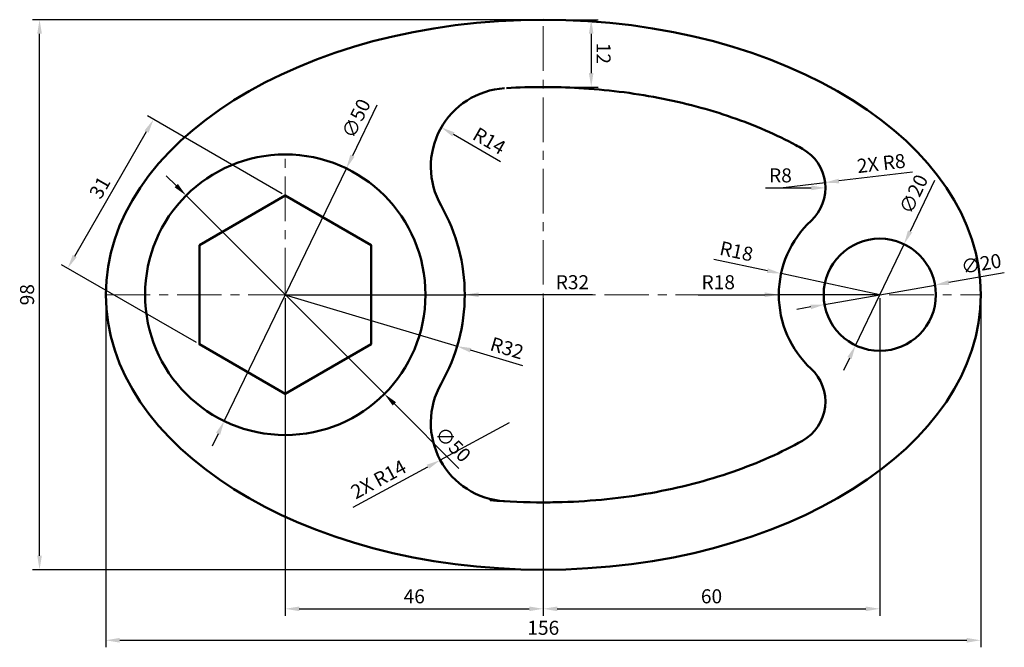
# Model space of a CAD drawing. Units: millimetres. Extents: x 1633 to 1808, y 1205 to 1317.
import ezdxf

# ---------------------------------------------------------------- set-up
doc = ezdxf.new("R2010")
doc.units = ezdxf.units.MM
doc.linetypes.add('CENTER', pattern=[50.8, 31.75, -6.35, 6.35, -6.35])
for name, color, linetype, lineweight in [('M-CNTR', 4, 'CENTER', 18), ('M-DIMS', 2, 'Continuous', 25), ('M-OUTL', 7, 'Continuous', 50)]:
    doc.layers.add(name, color=color, linetype=linetype, lineweight=lineweight)
doc.styles.get("Standard").update_dxf_attribs({"font": 'arial.ttf'})
doc.dimstyles.new('ISO-25', dxfattribs={"dimtxt": 2.5, "dimasz": 2.5, "dimexe": 1.25, "dimexo": 0.625, "dimtad": 1, "dimtxsty": 'Standard', "dimcen": 2.5, "dimadec": 0, "dimazin": 0, "dimtfac": 1, "dimtmove": 0, "dimatfit": 3, "dimfxl": 1, "dimarcsym": 0})

# ---------------------------------------------------------------- blocks, each defined once
blk = doc.blocks.new('*D1')
at = {"layer": 'Defpoints', "color": 0, "transparency": 16777216}
for p in [(1680.07, 1267.86), (1726.07, 1267.86), (1726.07, 1211.9)]:
    blk.add_point(p, dxfattribs=at)
at = {"layer": 'M-DIMS', "color": 0, "lineweight": -2, "transparency": 16777216}
for p, q in [((1680.07, 1267.23), (1680.07, 1210.65)), ((1726.07, 1267.23), (1726.07, 1210.65)), ((1682.57, 1211.9), (1723.57, 1211.9))]:
    blk.add_line(p, q, dxfattribs=at)
at = {"layer": 'M-DIMS', "color": 0, "transparency": 16777216}
for points in [[(1682.57, 1212.31), (1682.57, 1211.48), (1680.07, 1211.9)], [(1723.57, 1212.31), (1723.57, 1211.48), (1726.07, 1211.9)]]:
    blk.add_solid(points, dxfattribs=at)
at = {"layer": 'M-DIMS', "color": 0, "transparency": 16777216, "insert": (1703.07, 1213.8), "char_height": 2.5, "attachment_point": 5}
blk.add_mtext('46', dxfattribs=at)
blk = doc.blocks.new('*D2')
at = {"layer": 'Defpoints', "color": 0, "transparency": 16777216}
for p in [(1726.07, 1267.86), (1786.07, 1267.86), (1786.07, 1211.9)]:
    blk.add_point(p, dxfattribs=at)
at = {"layer": 'M-DIMS', "color": 0, "lineweight": -2, "transparency": 16777216}
for p, q in [((1726.07, 1267.23), (1726.07, 1210.65)), ((1786.07, 1267.23), (1786.07, 1210.65)), ((1728.57, 1211.9), (1783.57, 1211.9))]:
    blk.add_line(p, q, dxfattribs=at)
at = {"layer": 'M-DIMS', "color": 0, "transparency": 16777216}
for points in [[(1728.57, 1212.31), (1728.57, 1211.48), (1726.07, 1211.9)], [(1783.57, 1212.31), (1783.57, 1211.48), (1786.07, 1211.9)]]:
    blk.add_solid(points, dxfattribs=at)
at = {"layer": 'M-DIMS', "color": 0, "transparency": 16777216, "insert": (1756.07, 1213.8), "char_height": 2.5, "attachment_point": 5}
blk.add_mtext('60', dxfattribs=at)
blk = doc.blocks.new('*D3')
at = {"layer": 'Defpoints', "color": 0, "transparency": 16777216}
for p in [(1648.07, 1267.86), (1804.07, 1267.86), (1804.07, 1206.29)]:
    blk.add_point(p, dxfattribs=at)
at = {"layer": 'M-DIMS', "color": 0, "lineweight": -2, "transparency": 16777216}
for p, q in [((1648.07, 1267.23), (1648.07, 1205.04)), ((1804.07, 1267.23), (1804.07, 1205.04)), ((1650.57, 1206.29), (1801.57, 1206.29))]:
    blk.add_line(p, q, dxfattribs=at)
at = {"layer": 'M-DIMS', "color": 0, "transparency": 16777216}
for points in [[(1650.57, 1206.71), (1650.57, 1205.87), (1648.07, 1206.29)], [(1801.57, 1206.71), (1801.57, 1205.87), (1804.07, 1206.29)]]:
    blk.add_solid(points, dxfattribs=at)
at = {"layer": 'M-DIMS', "color": 0, "transparency": 16777216, "insert": (1726.07, 1208.19), "char_height": 2.5, "attachment_point": 5}
blk.add_mtext('156', dxfattribs=at)
blk = doc.blocks.new('*D4')
at = {"layer": 'Defpoints', "color": 0, "transparency": 16777216}
for p in [(1636.26, 1316.86), (1726.07, 1316.86), (1726.07, 1218.86)]:
    blk.add_point(p, dxfattribs=at)
at = {"layer": 'M-DIMS', "color": 0, "lineweight": -2, "transparency": 16777216}
for p, q in [((1725.45, 1316.86), (1635.01, 1316.86)), ((1636.26, 1221.36), (1636.26, 1314.36)), ((1725.45, 1218.86), (1635.01, 1218.86))]:
    blk.add_line(p, q, dxfattribs=at)
at = {"layer": 'M-DIMS', "color": 0, "transparency": 16777216}
for points in [[(1635.85, 1314.36), (1636.68, 1314.36), (1636.26, 1316.86)], [(1635.85, 1221.36), (1636.68, 1221.36), (1636.26, 1218.86)]]:
    blk.add_solid(points, dxfattribs=at)
at = {"layer": 'M-DIMS', "color": 0, "transparency": 16777216, "insert": (1634.36, 1267.86), "char_height": 2.5, "attachment_point": 5, "rotation": 90}
blk.add_mtext('98', dxfattribs=at)
blk = doc.blocks.new('*D5')
at = {"layer": 'Defpoints', "color": 0, "transparency": 16777216}
for p in [(1656.59, 1299.09), (1680.07, 1285.53), (1664.77, 1259.02)]:
    blk.add_point(p, dxfattribs=at)
at = {"layer": 'M-DIMS', "color": 0, "lineweight": -2, "transparency": 16777216}
for p, q in [((1679.53, 1285.84), (1655.5, 1299.71)), ((1642.53, 1274.75), (1655.34, 1296.92)), ((1664.23, 1259.33), (1640.2, 1273.21))]:
    blk.add_line(p, q, dxfattribs=at)
at = {"layer": 'M-DIMS', "color": 0, "transparency": 16777216}
for points in [[(1654.98, 1297.13), (1655.7, 1296.72), (1656.59, 1299.09)], [(1642.17, 1274.95), (1642.89, 1274.54), (1641.28, 1272.58)]]:
    blk.add_solid(points, dxfattribs=at)
at = {"layer": 'M-DIMS', "color": 0, "transparency": 16777216, "insert": (1647.29, 1286.79), "char_height": 2.5, "attachment_point": 5, "rotation": 60}
blk.add_mtext('31', dxfattribs=at)
blk = doc.blocks.new('*D6')
at = {"layer": 'Defpoints', "color": 0, "transparency": 16777216}
for p in [(1707.89, 1297.67), (1720.02, 1290.67)]:
    blk.add_point(p, dxfattribs=at)
at = {"layer": 'M-DIMS', "color": 0, "lineweight": -2, "transparency": 16777216}
blk.add_line((1718.47, 1291.56), (1710.06, 1296.42), dxfattribs=at)
at = {"layer": 'M-DIMS', "color": 0, "transparency": 16777216}
blk.add_solid([(1710.26, 1296.78), (1709.85, 1296.06), (1707.89, 1297.67)], dxfattribs=at)
at = {"layer": 'M-DIMS', "color": 0, "transparency": 16777216, "insert": (1716.29, 1294.99), "char_height": 2.5, "attachment_point": 5, "rotation": 330.0121}
blk.add_mtext('R14', dxfattribs=at)
blk = doc.blocks.new('*D7')
at = {"layer": 'Defpoints', "color": 0, "transparency": 16777216}
for p in [(1680.07, 1267.86), (1710.73, 1258.68)]:
    blk.add_point(p, dxfattribs=at)
at = {"layer": 'M-DIMS', "color": 0, "lineweight": -2, "transparency": 16777216}
for p, q in [((1680.07, 1267.86), (1710.73, 1258.68)), ((1722.41, 1255.18), (1713.12, 1257.96))]:
    blk.add_line(p, q, dxfattribs=at)
at = {"layer": 'M-DIMS', "color": 0, "transparency": 16777216}
blk.add_solid([(1713.24, 1258.36), (1713, 1257.56), (1710.73, 1258.68)], dxfattribs=at)
at = {"layer": 'M-DIMS', "color": 0, "transparency": 16777216, "insert": (1719.51, 1258.04), "char_height": 2.5, "attachment_point": 5, "rotation": 343.3331}
blk.add_mtext('R32', dxfattribs=at)
blk = doc.blocks.new('*D8')
at = {"layer": 'Defpoints', "color": 0, "transparency": 16777216}
for p in [(1768.36, 1286.89), (1776.36, 1286.89)]:
    blk.add_point(p, dxfattribs=at)
at = {"layer": 'M-DIMS', "color": 0, "lineweight": -2, "transparency": 16777216}
blk.add_line((1765.72, 1286.89), (1773.86, 1286.89), dxfattribs=at)
at = {"layer": 'M-DIMS', "color": 0, "transparency": 16777216}
blk.add_solid([(1773.86, 1287.31), (1773.86, 1286.48), (1776.36, 1286.89)], dxfattribs=at)
at = {"layer": 'M-DIMS', "color": 0, "transparency": 16777216, "insert": (1768.36, 1288.8), "char_height": 2.5, "attachment_point": 5}
blk.add_mtext('R8', dxfattribs=at)
blk = doc.blocks.new('*D9')
at = {"layer": 'Defpoints', "color": 0, "transparency": 16777216}
for p in [(1768.47, 1271.63), (1786.07, 1267.86)]:
    blk.add_point(p, dxfattribs=at)
at = {"layer": 'M-DIMS', "color": 0, "lineweight": -2, "transparency": 16777216}
for p, q in [((1756.51, 1274.19), (1766.03, 1272.15)), ((1786.07, 1267.86), (1768.47, 1271.63))]:
    blk.add_line(p, q, dxfattribs=at)
at = {"layer": 'M-DIMS', "color": 0, "transparency": 16777216}
blk.add_solid([(1766.11, 1272.56), (1765.94, 1271.74), (1768.47, 1271.63)], dxfattribs=at)
at = {"layer": 'M-DIMS', "color": 0, "transparency": 16777216, "insert": (1760.45, 1275.29), "char_height": 2.5, "attachment_point": 5, "rotation": 347.9168}
blk.add_mtext('R18', dxfattribs=at)
blk = doc.blocks.new('*D10')
at = {"layer": 'Defpoints', "color": 0, "transparency": 16777216}
for p in [(1790.39, 1276.88), (1781.75, 1258.84)]:
    blk.add_point(p, dxfattribs=at)
at = {"layer": 'M-DIMS', "color": 0, "lineweight": -2, "transparency": 16777216}
for p, q in [((1795.81, 1288.19), (1791.47, 1279.13)), ((1781.75, 1258.84), (1790.39, 1276.88)), ((1780.67, 1256.58), (1779.59, 1254.33))]:
    blk.add_line(p, q, dxfattribs=at)
at = {"layer": 'M-DIMS', "color": 0, "transparency": 16777216}
for points in [[(1791.1, 1279.31), (1791.85, 1278.95), (1790.39, 1276.88)], [(1780.3, 1256.76), (1781.05, 1256.4), (1781.75, 1258.84)]]:
    blk.add_solid(points, dxfattribs=at)
at = {"layer": 'M-DIMS', "color": 0, "transparency": 16777216, "insert": (1792.4, 1285.64), "char_height": 2.5, "attachment_point": 5, "rotation": 64.4044}
blk.add_mtext('∅20', dxfattribs=at)
blk = doc.blocks.new('*D11')
at = {"layer": 'Defpoints', "color": 0, "transparency": 16777216}
for p in [(1726.07, 1316.86), (1726.07, 1304.86), (1734.62, 1304.86)]:
    blk.add_point(p, dxfattribs=at)
at = {"layer": 'M-DIMS', "color": 0, "lineweight": -2, "transparency": 16777216}
for p, q in [((1726.7, 1316.86), (1735.87, 1316.86)), ((1734.62, 1314.36), (1734.62, 1307.36)), ((1726.7, 1304.86), (1735.87, 1304.86))]:
    blk.add_line(p, q, dxfattribs=at)
at = {"layer": 'M-DIMS', "color": 0, "transparency": 16777216}
for points in [[(1735.03, 1314.36), (1734.2, 1314.36), (1734.62, 1316.86)], [(1735.03, 1307.36), (1734.2, 1307.36), (1734.62, 1304.86)]]:
    blk.add_solid(points, dxfattribs=at)
at = {"layer": 'M-DIMS', "color": 0, "transparency": 16777216, "insert": (1736.5, 1310.86), "char_height": 2.5, "attachment_point": 5, "rotation": 270.0011}
blk.add_mtext('12', dxfattribs=at)
blk = doc.blocks.new('*D12')
at = {"layer": 'Defpoints', "color": 0, "transparency": 16777216}
for p in [(1690.96, 1290.36), (1669.19, 1245.35)]:
    blk.add_point(p, dxfattribs=at)
at = {"layer": 'M-DIMS', "color": 0, "lineweight": -2, "transparency": 16777216}
for p, q in [((1696.42, 1301.65), (1692.05, 1292.61)), ((1669.19, 1245.35), (1690.96, 1290.36)), ((1668.1, 1243.1), (1667.01, 1240.85))]:
    blk.add_line(p, q, dxfattribs=at)
at = {"layer": 'M-DIMS', "color": 0, "transparency": 16777216}
for points in [[(1691.67, 1292.8), (1692.42, 1292.43), (1690.96, 1290.36)], [(1667.72, 1243.28), (1668.47, 1242.92), (1669.19, 1245.35)]]:
    blk.add_solid(points, dxfattribs=at)
at = {"layer": 'M-DIMS', "color": 0, "transparency": 16777216, "insert": (1693, 1299.12), "char_height": 2.5, "attachment_point": 5, "rotation": 64.1877}
blk.add_mtext('∅50', dxfattribs=at)
blk = doc.blocks.new('*D13')
at = {"layer": 'Defpoints', "color": 0, "transparency": 16777216}
for p in [(1662.39, 1285.54), (1697.75, 1250.18)]:
    blk.add_point(p, dxfattribs=at)
at = {"layer": 'M-DIMS', "color": 0, "lineweight": -2, "transparency": 16777216}
for p, q in [((1660.63, 1287.3), (1658.86, 1289.07)), ((1662.39, 1285.54), (1697.75, 1250.18)), ((1711.02, 1236.91), (1699.52, 1248.41))]:
    blk.add_line(p, q, dxfattribs=at)
at = {"layer": 'M-DIMS', "color": 0, "transparency": 16777216}
for points in [[(1660.92, 1287.6), (1660.33, 1287.01), (1662.39, 1285.54)], [(1699.81, 1248.71), (1699.22, 1248.12), (1697.75, 1250.18)]]:
    blk.add_solid(points, dxfattribs=at)
at = {"layer": 'M-DIMS', "color": 0, "transparency": 16777216, "insert": (1709.75, 1240.97), "char_height": 2.5, "attachment_point": 5, "rotation": 315}
blk.add_mtext('∅50', dxfattribs=at)
blk = doc.blocks.new('*D14')
at = {"layer": 'Defpoints', "color": 0, "transparency": 16777216}
for p in [(1795.92, 1269.59), (1776.22, 1266.12)]:
    blk.add_point(p, dxfattribs=at)
at = {"layer": 'M-DIMS', "color": 0, "lineweight": -2, "transparency": 16777216}
for p, q in [((1808.27, 1271.77), (1798.38, 1270.03)), ((1776.22, 1266.12), (1795.92, 1269.59)), ((1773.76, 1265.69), (1771.3, 1265.25))]:
    blk.add_line(p, q, dxfattribs=at)
at = {"layer": 'M-DIMS', "color": 0, "transparency": 16777216}
for points in [[(1798.31, 1270.44), (1798.45, 1269.62), (1795.92, 1269.59)], [(1773.69, 1266.1), (1773.83, 1265.28), (1776.22, 1266.12)]]:
    blk.add_solid(points, dxfattribs=at)
at = {"layer": 'M-DIMS', "color": 0, "transparency": 16777216, "insert": (1804.22, 1273.06), "char_height": 2.5, "attachment_point": 5, "rotation": 9.9987}
blk.add_mtext('∅20', dxfattribs=at)
blk = doc.blocks.new('*D15')
at = {"layer": 'Defpoints', "color": 0, "transparency": 16777216}
for p in [(1680.07, 1267.86), (1712.07, 1267.86)]:
    blk.add_point(p, dxfattribs=at)
at = {"layer": 'M-DIMS', "color": 0, "lineweight": -2, "transparency": 16777216}
for p, q in [((1680.07, 1267.86), (1712.07, 1267.86)), ((1734.87, 1267.86), (1714.57, 1267.86))]:
    blk.add_line(p, q, dxfattribs=at)
at = {"layer": 'M-DIMS', "color": 0, "transparency": 16777216}
blk.add_solid([(1714.57, 1268.27), (1714.57, 1267.44), (1712.07, 1267.86)], dxfattribs=at)
at = {"layer": 'M-DIMS', "color": 0, "transparency": 16777216, "insert": (1731.27, 1269.76), "char_height": 2.5, "attachment_point": 5, "rotation": 0.0004}
blk.add_mtext('R32', dxfattribs=at)
blk = doc.blocks.new('*D16')
at = {"layer": 'Defpoints', "color": 0, "transparency": 16777216}
for p in [(1768.07, 1267.86), (1786.07, 1267.86)]:
    blk.add_point(p, dxfattribs=at)
at = {"layer": 'M-DIMS', "color": 0, "lineweight": -2, "transparency": 16777216}
for p, q in [((1753.66, 1267.86), (1765.57, 1267.86)), ((1786.07, 1267.86), (1768.07, 1267.86))]:
    blk.add_line(p, q, dxfattribs=at)
at = {"layer": 'M-DIMS', "color": 0, "transparency": 16777216}
blk.add_solid([(1765.57, 1268.27), (1765.57, 1267.44), (1768.07, 1267.86)], dxfattribs=at)
at = {"layer": 'M-DIMS', "color": 0, "transparency": 16777216, "insert": (1757.27, 1269.76), "char_height": 2.5, "attachment_point": 5, "rotation": 359.9993}
blk.add_mtext('R18', dxfattribs=at)
blk = doc.blocks.new('*D17')
at = {"layer": 'Defpoints', "color": 0, "transparency": 16777216}
for p in [(1720.02, 1245.05), (1707.7, 1238.39)]:
    blk.add_point(p, dxfattribs=at)
at = {"layer": 'M-DIMS', "color": 0, "lineweight": -2, "transparency": 16777216}
for p, q in [((1720.02, 1245.05), (1707.7, 1238.39)), ((1692.19, 1230.02), (1705.5, 1237.21))]:
    blk.add_line(p, q, dxfattribs=at)
at = {"layer": 'M-DIMS', "color": 0, "transparency": 16777216}
blk.add_solid([(1705.3, 1237.57), (1705.7, 1236.84), (1707.7, 1238.39)], dxfattribs=at)
at = {"layer": 'M-DIMS', "color": 0, "transparency": 16777216, "insert": (1696.85, 1234.68), "char_height": 2.5, "attachment_point": 5, "rotation": 28.3624}
blk.add_mtext('2X R14', dxfattribs=at)
blk = doc.blocks.new('*D18')
at = {"layer": 'Defpoints', "color": 0, "transparency": 16777216}
for p in [(1768.36, 1286.89), (1776.31, 1287.83)]:
    blk.add_point(p, dxfattribs=at)
at = {"layer": 'M-DIMS', "color": 0, "lineweight": -2, "transparency": 16777216}
for p, q in [((1791.9, 1289.68), (1778.79, 1288.13)), ((1768.36, 1286.89), (1776.31, 1287.83))]:
    blk.add_line(p, q, dxfattribs=at)
at = {"layer": 'M-DIMS', "color": 0, "transparency": 16777216}
blk.add_solid([(1778.74, 1288.54), (1778.84, 1287.71), (1776.31, 1287.83)], dxfattribs=at)
at = {"layer": 'M-DIMS', "color": 0, "transparency": 16777216, "insert": (1786.36, 1290.94), "char_height": 2.5, "attachment_point": 5, "rotation": 6.7445}
blk.add_mtext('2X R8', dxfattribs=at)

msp = doc.modelspace()

# ---------------------------------------------------------------- linework, layer by layer
at = {"layer": 'M-CNTR', "ltscale": 0.25, "transparency": 33554534}
for p, q in [((1726.072, 1218.858), (1726.072, 1316.858)), ((1680.072, 1242.858), (1680.072, 1292.858)), ((1648.072, 1267.858), (1804.072, 1267.858))]:
    msp.add_line(p, q, dxfattribs=at)
at = {"layer": 'M-OUTL'}
msp.add_line((1716.61, 1231.258), (1716.61, 1231.467), dxfattribs=at)
msp.add_lwpolyline([(1664.767, 1276.694), (1664.767, 1259.021), (1680.072, 1250.185), (1695.377, 1259.021), (1695.377, 1276.694), (1680.072, 1285.531)], close=True, dxfattribs=at)
for centre, radius in [((1680.072, 1267.858), 25), ((1786.072, 1267.858), 10)]:
    msp.add_circle(centre, radius, dxfattribs=at)
for centre, radius, start, end in [((1720.017, 1290.67), 14, 93.54668, 209.73095), ((1768.363, 1286.894), 8, 312.93059, 60.56486), ((1680.072, 1267.858), 32, 330.2696, 29.73095), ((1786.072, 1267.858), 18, 132.93059, 227.0695), ((1768.363, 1248.821), 8, 299.43079, 47.0695), ((1720.017, 1245.045), 14, 150.2696, 266.45457)]:
    msp.add_arc(centre, radius, start, end, dxfattribs=at)
msp.add_ellipse((1726.072, 1267.858), major_axis=(78, 0), ratio=0.6282051, dxfattribs=at)
for points, knots in [([(1772.295, 1293.862), (1771.91, 1294.079), (1771.521, 1294.293), (1767.671, 1296.365), (1763.833, 1298.039), (1755.583, 1300.886), (1751.171, 1302.058), (1741.998, 1303.817), (1737.237, 1304.404), (1730.312, 1304.798), (1728.192, 1304.858), (1726.072, 1304.857), (1723.89, 1304.857), (1721.708, 1304.794), (1719.525, 1304.667)], [0.83901384, 0.83901384, 0.83901384, 0.83901384, 0.8625381, 0.8625381, 1.06853493, 1.06853493, 1.27453175, 1.27453175, 1.48052858, 1.48052858, 1.57079638, 1.57079638, 1.57079638, 1.66370971, 1.66370971, 1.66370971, 1.66370971]), ([(1716.61, 1231.258), (1719.764, 1230.992), (1722.918, 1230.858), (1726.072, 1230.858), (1727.191, 1230.858), (1728.309, 1230.875), (1734.789, 1231.069), (1740.116, 1231.617), (1750.37, 1233.443), (1755.296, 1234.721), (1764.402, 1237.883), (1768.586, 1239.761), (1772.294, 1241.854)], [4.57809286, 4.57809286, 4.57809286, 4.57809286, 4.71238878, 4.71238878, 4.71238878, 4.76001282, 4.76001282, 4.98864883, 4.98864883, 5.21728484, 5.21728484, 5.4441605, 5.4441605, 5.4441605, 5.4441605])]:
    msp.add_open_spline(points, degree=3, knots=knots, dxfattribs=at)

# ---------------------------------------------------------------- dimensions: what is measured, and where the dimension line sits
at = {"layer": 'M-DIMS'}
dim = msp.add_linear_dim(base=(1636.263, 1316.858), p1=(1726.072, 1218.858), p2=(1726.072, 1316.858), angle=90, dimstyle='ISO-25', override={"dimclrd": 0, "dimclre": 0, "dimclrt": 0}, dxfattribs=at)
dim.commit()
dim.dimension.update_dxf_attribs({"geometry": '*D4', "text_midpoint": (1634.362, 1267.858)})
for p1, p2, distance, override, picture, middle in [((1726.072, 1316.858), (1726.072, 1304.857), 8.543, {"dimclrd": 0, "dimclre": 0, "dimclrt": 0}, '*D11', (1736.495, 1310.858)), ((1664.767, 1259.021), (1680.072, 1285.531), 27.118, {"dimdec": 0, "dimclrd": 0, "dimclre": 0, "dimclrt": 0}, '*D5', (1647.287, 1286.786))]:
    dim = msp.add_aligned_dim(p1=p1, p2=p2, distance=distance, dimstyle='ISO-25', override=override, dxfattribs=at)
    dim.commit()
    dim.dimension.update_dxf_attribs({"geometry": picture, "text_midpoint": middle})
for p1, p2, override, picture, middle in [((1669.187, 1245.352), (1690.958, 1290.363), {"dimclrd": 0, "dimclre": 0, "dimclrt": 0}, '*D12', (1693.002, 1299.118)), ((1781.752, 1258.839), (1790.392, 1276.876), {"dimclrd": 0, "dimclre": 0, "dimclrt": 0}, '*D10', (1792.404, 1285.639)), ((1776.224, 1266.122), (1795.92, 1269.594), {"dimdec": 0, "dimlfac": 1, "dimrnd": 0, "dimzin": 0, "dimdsep": 46, "dimlunit": 2}, '*D14', (1804.558, 1271.117))]:
    dim = msp.add_diameter_dim_2p(p1=p1, p2=p2, dimstyle='ISO-25', override=override, dxfattribs=at)
    dim.commit()
    dim.dimension.update_dxf_attribs({"geometry": picture, "text_midpoint": middle})
for center, mpoint, override, picture, middle in [((1720.017, 1290.67), (1707.891, 1297.668), {"dimclrd": 0, "dimclre": 0, "dimclrt": 0}, '*D6', (1715.346, 1293.366)), ((1768.363, 1286.894), (1776.363, 1286.894), {"dimclrd": 0, "dimclre": 0, "dimclrt": 0}, '*D8', (1768.363, 1286.894)), ((1680.072, 1267.858), (1712.072, 1267.858), {"dimdec": 0, "dimlfac": 1, "dimrnd": 0, "dimzin": 0, "dimdsep": 46, "dimlunit": 2}, '*D15', (1731.272, 1267.858)), ((1786.072, 1267.858), (1768.072, 1267.858), {"dimdec": 0, "dimlfac": 1, "dimrnd": 0, "dimzin": 0, "dimdsep": 46, "dimlunit": 2}, '*D16', (1757.272, 1267.858))]:
    dim = msp.add_radius_dim(center=center, mpoint=mpoint, dimstyle='ISO-25', override=override, dxfattribs=at)
    dim.commit()
    dim.dimension.update_dxf_attribs({"geometry": picture, "text_midpoint": middle, "dimtype": 164})
for center, mpoint, picture, middle in [((1768.363, 1286.894), (1776.308, 1287.834), '*D18', (1786.363, 1290.938)), ((1720.017, 1245.045), (1707.698, 1238.395), '*D17', (1696.848, 1234.675))]:
    dim = msp.add_radius_dim(center=center, mpoint=mpoint, text='2X <>', dimstyle='ISO-25', override={"dimdec": 0, "dimlfac": 1, "dimrnd": 0, "dimzin": 0, "dimdsep": 46, "dimlunit": 2}, dxfattribs=at)
    dim.commit()
    dim.dimension.update_dxf_attribs({"geometry": picture, "text_midpoint": middle})
dim = msp.add_diameter_dim_2p(p1=(1662.395, 1285.535), p2=(1697.75, 1250.18), dimstyle='ISO-25', override={"dimdec": 0, "dimlfac": 1, "dimrnd": 0, "dimzin": 0, "dimdsep": 46, "dimlunit": 2}, dxfattribs=at)
dim.commit()
dim.dimension.update_dxf_attribs({"geometry": '*D13', "text_midpoint": (1708.356, 1239.574), "dimtype": 163})
for center, mpoint, picture, middle in [((1786.072, 1267.858), (1768.471, 1271.626), '*D9', (1760.445, 1275.288)), ((1680.072, 1267.858), (1710.728, 1258.68), '*D7', (1719.511, 1258.036))]:
    dim = msp.add_radius_dim(center=center, mpoint=mpoint, dimstyle='ISO-25', override={"dimclrd": 0, "dimclre": 0, "dimclrt": 0}, dxfattribs=at)
    dim.commit()
    dim.dimension.update_dxf_attribs({"geometry": picture, "text_midpoint": middle})
for base, p1, p2, picture, middle in [((1804.072, 1206.291), (1648.072, 1267.858), (1804.072, 1267.858), '*D3', (1726.072, 1208.192)), ((1726.072, 1211.895), (1680.072, 1267.858), (1726.072, 1267.858), '*D1', (1703.072, 1213.797)), ((1786.072, 1211.895), (1726.072, 1267.858), (1786.072, 1267.858), '*D2', (1756.072, 1213.797))]:
    dim = msp.add_linear_dim(base=base, p1=p1, p2=p2, dimstyle='ISO-25', override={"dimclrd": 0, "dimclre": 0, "dimclrt": 0}, dxfattribs=at)
    dim.commit()
    dim.dimension.update_dxf_attribs({"geometry": picture, "text_midpoint": middle})

doc.saveas('drawing.dxf')
